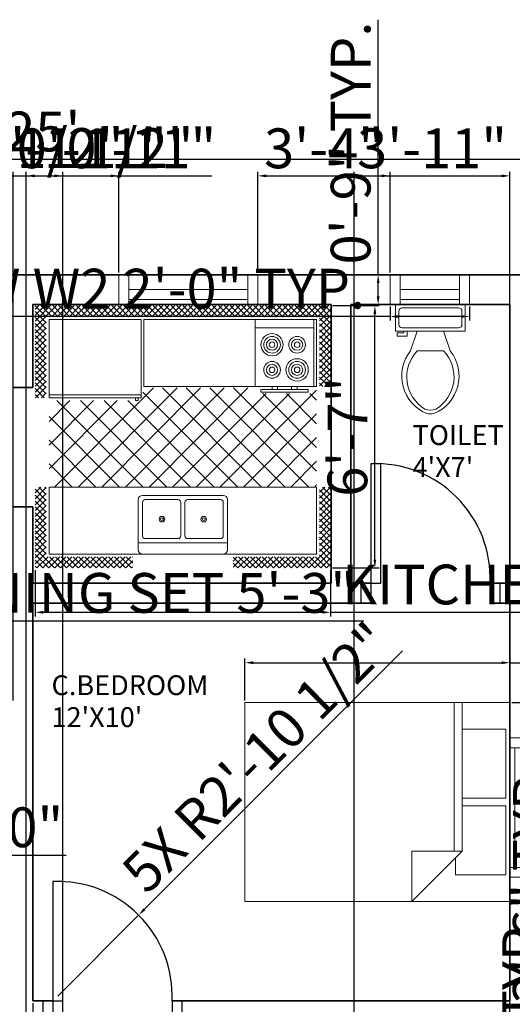
# Model space of a CAD drawing. Units: inches. Extents: x 2011 to 2548, y 530 to 1188.
# Tile 4 of 5: x 2220 to 2368, y 891 to 1188. Entities that reach past the tile are written whole.
import ezdxf

# ---------------------------------------------------------------- set-up
doc = ezdxf.new("R2010")
doc.units = ezdxf.units.IN
for name, color, linetype, lineweight in [('A-ANNO-DIMS', 2, 'Continuous', 18), ('A-AREA-IDEN', 7, 'Continuous', 25), ('A-DOOR', 3, 'Continuous', 25), ('A-FLOR-FIXT', 9, 'Continuous', 18), ('A-FURN', 8, 'Continuous', 18), ('A-GLAZ', 4, 'Continuous', 18), ('A-WALL', 7, 'Continuous', 35)]:
    doc.layers.add(name, color=color, linetype=linetype, lineweight=lineweight)
doc.styles.get("Standard").update_dxf_attribs({"font": 'arial.ttf'})
doc.dimstyles.new('ISO-25', dxfattribs={"dimtxt": 12, "dimasz": 2.5, "dimexe": 1.25, "dimexo": 0.625, "dimtad": 1, "dimdec": 1, "dimlunit": 3, "dimtxsty": 'Standard', "dimcen": 2.5, "dimadec": 0, "dimazin": 0, "dimtfac": 1, "dimtdec": 1, "dimtmove": 0, "dimatfit": 3, "dimfxl": 1, "dimarcsym": 0})

# ---------------------------------------------------------------- blocks, each defined once
blk = doc.blocks.new('Kitchen Layout - 7 x 8 ft')
for p, q in [((-5, 81.32), (2.68, 89)), ((-5, 83.44), (0.56, 89)), ((-5, 85.56), (-1.56, 89)), ((-5, 87.68), (-3.68, 89)), ((-1, 84.97), (-5, 88.97)), ((1.09, 85), (-2.91, 89)), ((3.21, 85), (-0.79, 89)), ((0.81, 85), (4.81, 89)), ((5.34, 85), (1.34, 89)), ((2.93, 85), (6.93, 89)), ((7.46, 85), (3.46, 89)), ((5.05, 85), (9.05, 89)), ((9.58, 85), (5.58, 89)), ((7.17, 85), (11.17, 89)), ((11.7, 85), (7.7, 89)), ((9.29, 85), (13.29, 89)), ((13.82, 85), (9.82, 89)), ((11.41, 85), (15.41, 89)), ((15.94, 85), (11.94, 89)), ((13.53, 85), (17.53, 89)), ((18.06, 85), (14.06, 89)), ((15.65, 85), (19.65, 89)), ((20.18, 85), (16.18, 89)), ((17.78, 85), (21.78, 89)), ((22.31, 85), (18.31, 89)), ((19.9, 85), (23.9, 89)), ((24.43, 85), (20.43, 89)), ((22.02, 85), (26.02, 89)), ((26.55, 85), (22.55, 89)), ((24.14, 85), (28.14, 89)), ((28.67, 85), (24.67, 89)), ((26.26, 85), (30.26, 89)), ((30.79, 85), (26.79, 89)), ((28.38, 85), (32.38, 89)), ((32.91, 85), (28.91, 89)), ((30.5, 85), (34.5, 89)), ((35.03, 85), (31.03, 89)), ((32.63, 85), (36.63, 89)), ((37.16, 85), (33.16, 89)), ((34.75, 85), (38.75, 89)), ((39.28, 85), (35.28, 89)), ((36.87, 85), (40.87, 89)), ((41.4, 85), (37.4, 89)), ((38.99, 85), (42.99, 89)), ((43.52, 85), (39.52, 89)), ((41.11, 85), (45.11, 89)), ((45.64, 85), (41.64, 89)), ((43.23, 85), (47.23, 89)), ((47.76, 85), (43.76, 89)), ((45.35, 85), (49.35, 89)), ((49.88, 85), (45.88, 89)), ((47.47, 85), (51.47, 89)), ((52, 85), (48, 89)), ((49.6, 85), (53.6, 89)), ((54.13, 85), (50.13, 89)), ((51.72, 85), (55.72, 89)), ((56.25, 85), (52.25, 89)), ((53.84, 85), (57.84, 89)), ((58.37, 85), (54.37, 89)), ((55.96, 85), (59.96, 89)), ((60.49, 85), (56.49, 89)), ((58.08, 85), (62.08, 89)), ((62.61, 85), (58.61, 89)), ((60.2, 85), (64.2, 89)), ((64.73, 85), (60.73, 89)), ((62.32, 85), (66.32, 89)), ((66.85, 85), (62.85, 89)), ((64.45, 85), (68.45, 89)), ((68.97, 85), (64.97, 89)), ((66.57, 85), (70.57, 89)), ((71.1, 85), (67.1, 89)), ((68.69, 85), (72.69, 89)), ((73.22, 85), (69.22, 89)), ((70.81, 85), (74.81, 89)), ((75.34, 85), (71.34, 89)), ((72.93, 85), (76.93, 89)), ((77.46, 85), (73.46, 89)), ((75.05, 85), (79.05, 89)), ((79.58, 85), (75.58, 89)), ((77.17, 85), (81.17, 89)), ((81.7, 85), (77.7, 89)), ((79.29, 85), (83.29, 89)), ((83.82, 85), (79.82, 89)), ((81.42, 85), (85.42, 89)), ((85.95, 85), (81.95, 89)), ((83.54, 85), (87.54, 89)), ((88.07, 85), (84.07, 89)), ((85.66, 85), (89.66, 89)), ((90.19, 85), (86.19, 89)), ((87.78, 85), (91.78, 89)), ((92.31, 85), (88.31, 89)), ((89.9, 85), (93.9, 89)), ((94.43, 85), (90.43, 89)), ((92.02, 85), (96.02, 89)), ((96.55, 85), (92.55, 89)), ((94.14, 85), (98.14, 89)), ((101, 82.67), (94.67, 89)), ((96.27, 85), (100.27, 89)), ((101, 84.79), (96.79, 89)), ((101, 86.92), (98.92, 89)), ((-1, 82.85), (-5, 86.85)), ((-1, 80.73), (-5, 84.73)), ((97, 83.61), (101, 87.61)), ((97, 81.49), (101, 85.49)), ((-5, 79.19), (-1, 83.19)), ((-1, 78.61), (-5, 82.61)), ((34, 84), (96, 84)), ((34, 60), (34, 84)), ((96, 84), (96, 60)), ((101, 80.55), (97, 84.55)), ((97, 79.37), (101, 83.37)), ((101, 78.43), (97, 82.43)), ((97, 77.25), (101, 81.25)), ((-5, 77.07), (-1, 81.07)), ((-1, 76.49), (-5, 80.49)), ((-5, 74.95), (-1, 78.95)), ((-1, 74.36), (-5, 78.36)), ((74, 81), (95, 81)), ((101, 76.31), (97, 80.31)), ((97, 75.13), (101, 79.13)), ((101, 74.19), (97, 78.19)), ((-5, 72.83), (-1, 76.83)), ((-1, 72.24), (-5, 76.24)), ((-5, 70.71), (-1, 74.71)), ((-1, 70.12), (-5, 74.12)), ((97, 73.01), (101, 77.01)), ((101, 72.07), (97, 76.07)), ((97, 70.89), (101, 74.89)), ((-5, 68.59), (-1, 72.59)), ((-1, 68), (-5, 72)), ((101, 69.95), (97, 73.95)), ((97, 68.76), (101, 72.76)), ((101, 67.82), (97, 71.82)), ((97, 66.64), (101, 70.64)), ((-5, 66.47), (-1, 70.47)), ((-1, 65.88), (-5, 69.88)), ((-5, 64.35), (-1, 68.35)), ((-1, 63.76), (-5, 67.76)), ((101, 65.7), (97, 69.7)), ((97, 64.52), (101, 68.52)), ((101, 63.58), (97, 67.58)), ((-5, 62.22), (-1, 66.22)), ((-1, 61.64), (-5, 65.64)), ((-5, 60.1), (-1, 64.1)), ((97, 62.4), (101, 66.4)), ((101, 61.46), (97, 65.46)), ((97, 60.28), (101, 64.28)), ((-1, 59.52), (-5, 63.52)), ((-5, 57.98), (-1, 61.98)), ((-1, 57.39), (-5, 61.39)), ((96, 60), (34, 60)), ((80, 60), (80, 59)), ((82, 59), (82, 60)), ((87, 59), (87, 60)), ((89, 60), (89, 59)), ((100.34, 60), (97, 63.34)), ((98.22, 60), (97, 61.22)), ((98.84, 60), (101, 62.16)), ((100.96, 60), (101, 60.04)), ((-1.73, 56), (-5, 59.27)), ((-3.85, 56), (-5, 57.15)), ((-4.86, 56), (-1, 59.86)), ((-2.74, 56), (-1, 57.74)), ((0, 57), (33, 57)), ((10.4, 24), (45.9, 59.5)), ((18.88, 24), (54.38, 59.5)), ((27.37, 24), (62.87, 59.5)), ((33.03, 55.11), (37.41, 59.5)), ((67.71, 24), (33.68, 58.04)), ((35.85, 24), (71.35, 59.5)), ((76.2, 24), (40.7, 59.5)), ((44.34, 24), (77.84, 57.5)), ((84.68, 24), (49.18, 59.5)), ((52.82, 24), (86.32, 57.5)), ((93.17, 24), (57.67, 59.5)), ((61.31, 24), (96, 58.69)), ((96, 29.65), (66.15, 59.5)), ((96, 38.14), (76.64, 57.5)), ((96, 46.63), (85.13, 57.5)), ((96, 55.11), (93.57, 57.54)), ((0, 30.57), (24.43, 55)), ((0, 39.06), (15.94, 55)), ((0, 47.54), (7.46, 55)), ((1.91, 24), (32.91, 55)), ((33.77, 24), (2.77, 55)), ((42.26, 24), (11.26, 55)), ((50.74, 24), (19.74, 55)), ((59.23, 24), (28.23, 55)), ((31, 55), (31, 56)), ((32, 55), (31, 55)), ((32, 56), (32, 55)), ((69.79, 24), (96, 50.21)), ((25.29, 24), (0, 49.29)), ((16.8, 24), (0, 40.8)), ((78.28, 24), (96, 41.72)), ((8.32, 24), (0, 32.32)), ((86.76, 24), (96, 33.24)), ((95.25, 24), (96, 24.75)), ((-5, 21.92), (-2.92, 24)), ((-5, 19.8), (-1, 23.8)), ((-1, 19.21), (-5, 23.21)), ((-5, 17.68), (-1, 21.68)), ((-1, 21.33), (-3.67, 24)), ((-1, 23.45), (-1.55, 24)), ((0, 24), (96, 24)), ((0, 0), (0, 24)), ((96, 24), (96, 0)), ((97, 22.1), (98.9, 24)), ((97, 19.97), (101, 23.97)), ((101, 19.03), (97, 23.03)), ((97, 17.85), (101, 21.85)), ((101, 21.16), (98.16, 24)), ((101, 23.28), (100.28, 24)), ((-1, 17.09), (-5, 21.09)), ((-5, 15.55), (-1, 19.55)), ((-1, 14.97), (-5, 18.97)), ((47.25, 6.5), (47.25, 18.5)), ((48.75, 18.5), (48.75, 6.5)), ((101, 16.91), (97, 20.91)), ((97, 15.73), (101, 19.73)), ((101, 14.79), (97, 18.79)), ((-5, 13.43), (-1, 17.43)), ((-1, 12.85), (-5, 16.85)), ((-5, 11.31), (-1, 15.31)), ((-1, 10.73), (-5, 14.73)), ((97, 13.61), (101, 17.61)), ((101, 12.67), (97, 16.67)), ((97, 11.49), (101, 15.49)), ((101, 10.55), (97, 14.55)), ((-5, 9.19), (-1, 13.19)), ((-1, 8.6), (-5, 12.6)), ((-5, 7.07), (-1, 11.07)), ((97, 9.37), (101, 13.37)), ((101, 8.43), (97, 12.43)), ((97, 7.25), (101, 11.25)), ((-1, 6.48), (-5, 10.48)), ((-5, 4.95), (-1, 8.95)), ((-1, 4.36), (-5, 8.36)), ((101, 6.31), (97, 10.31)), ((97, 5.12), (101, 9.12)), ((101, 4.18), (97, 8.18)), ((-5, 2.83), (-1, 6.83)), ((-1, 2.24), (-5, 6.24)), ((-5, 0.71), (-1, 4.71)), ((-1, 0.12), (-5, 4.12)), ((64, 4), (32, 4)), ((97, 3), (101, 7)), ((101, 2.06), (97, 6.06)), ((97, 0.88), (101, 4.88)), ((101, -0.06), (97, 3.94)), ((-5, -1.42), (-1, 2.58)), ((2, -5), (-5, 2)), ((-5, -3.54), (-1, 0.46)), ((96, 0), (0, 0)), ((93.24, -5), (101, 2.76)), ((95.36, -5), (101, 0.64)), ((101, -2.18), (97, 1.82)), ((-0.12, -5), (-5, -0.12)), ((-2.25, -5), (-5, -2.25)), ((-4.34, -5), (-0.34, -1)), ((-2.22, -5), (1.78, -1)), ((-0.1, -5), (3.9, -1)), ((4.12, -5), (0.12, -1)), ((2.02, -5), (6.02, -1)), ((6.24, -5), (2.24, -1)), ((4.14, -5), (8.14, -1)), ((8.36, -5), (4.36, -1)), ((6.27, -5), (10.27, -1)), ((10.48, -5), (6.48, -1)), ((8.39, -5), (12.39, -1)), ((12.6, -5), (8.6, -1)), ((10.51, -5), (14.51, -1)), ((14.73, -5), (10.73, -1)), ((12.63, -5), (16.63, -1)), ((16.85, -5), (12.85, -1)), ((14.75, -5), (18.75, -1)), ((18.97, -5), (14.97, -1)), ((16.87, -5), (20.87, -1)), ((21.09, -5), (17.09, -1)), ((18.99, -5), (22.99, -1)), ((23.21, -5), (19.21, -1)), ((21.11, -5), (25.11, -1)), ((25.33, -5), (21.33, -1)), ((23.24, -5), (27.24, -1)), ((27.45, -5), (23.45, -1)), ((25.36, -5), (29.36, -1)), ((29.57, -5), (25.57, -1)), ((27.48, -5), (30, -2.48)), ((30, -3.3), (27.7, -1)), ((30, -1.18), (29.82, -1)), ((66, -2.54), (67.54, -1)), ((66, -4.66), (69.66, -1)), ((69.88, -5), (66, -1.12)), ((67.76, -5), (66, -3.24)), ((67.78, -5), (71.78, -1)), ((72, -5), (68, -1)), ((69.9, -5), (73.9, -1)), ((74.12, -5), (70.12, -1)), ((72.03, -5), (76.03, -1)), ((76.24, -5), (72.24, -1)), ((74.15, -5), (78.15, -1)), ((78.36, -5), (74.36, -1)), ((76.27, -5), (80.27, -1)), ((80.49, -5), (76.49, -1)), ((78.39, -5), (82.39, -1)), ((82.61, -5), (78.61, -1)), ((80.51, -5), (84.51, -1)), ((84.73, -5), (80.73, -1)), ((82.63, -5), (86.63, -1)), ((86.85, -5), (82.85, -1)), ((84.75, -5), (88.75, -1)), ((88.97, -5), (84.97, -1)), ((86.88, -5), (90.88, -1)), ((91.09, -5), (87.09, -1)), ((89, -5), (93, -1)), ((93.21, -5), (89.21, -1)), ((91.12, -5), (95.12, -1)), ((95.34, -5), (91.34, -1)), ((97.46, -5), (93.46, -1)), ((99.58, -5), (95.58, -1)), ((101, -4.3), (97, -0.3)), ((97.48, -5), (101, -1.48)), ((-4.37, -5), (-5, -4.37)), ((29.6, -5), (30, -4.6)), ((99.6, -5), (101, -3.6))]:
    blk.add_line(p, q)
for points in [[(0, 56), (0, 84), (33, 84), (33, 56)], [(74, 60), (74, 84), (95, 84), (95, 60)], [(76, 58), (76, 59), (93, 59), (93, 58)]]:
    blk.add_lwpolyline(points, close=True)
for points in [[(32, 1.5), (32, 19.5)], [(33.5, 21), (62.5, 21)], [(33.5, 6.5), (33.5, 18.5)], [(34.5, 19.5), (46.25, 19.5)], [(49.75, 19.5), (61.5, 19.5)], [(62.5, 18.5), (62.5, 6.5)], [(64, 19.5), (64, 1.5)], [(46.25, 5.5), (34.5, 5.5)], [(61.5, 5.5), (49.75, 5.5)], [(62.5, 0), (33.5, 0)]]:
    blk.add_lwpolyline(points)
for centre, radius in [((80, 75), 4), ((80, 75), 3), ((89, 75), 3), ((80, 75), 2), ((80, 75), 1), ((89, 75), 2), ((89, 75), 1), ((80, 66), 3), ((80, 66), 2), ((89, 66), 4), ((89, 66), 3), ((89, 66), 2), ((80, 66), 1), ((89, 66), 1), ((40.5, 12.5), 1), ((40.5, 12.5), 0.5), ((55.5, 12.5), 1), ((55.5, 12.5), 0.5)]:
    blk.add_circle(centre, radius)
for centre, radius, start, end in [((33.5, 19.5), 1.5, 90, 180), ((34.5, 18.5), 1, 90, 180), ((46.25, 18.5), 1, 0, 90), ((49.75, 18.5), 1, 90, 180), ((61.5, 18.5), 1, 0, 90), ((62.5, 19.5), 1.5, 0, 90), ((34.5, 6.5), 1, 180, 270), ((46.25, 6.5), 1, 270, 0), ((49.75, 6.5), 1, 180, 270), ((61.5, 6.5), 1, 270, 0), ((33.5, 1.5), 1.5, 180, 270), ((62.5, 1.5), 1.5, 270, 0)]:
    blk.add_arc(centre, radius, start, end)
blk = doc.blocks.new('Toilet - top')
for p, q in [((9.5, -6), (9.5, -2)), ((-10, -8.5), (-8, -8.5)), ((-10, -9.5), (-10, -8.5)), ((-8, -8.5), (-8, -8)), ((-7, -8), (-7, -9.5)), ((-4, -8), (-6, -14)), ((4, -8), (6, -14)), ((-7, -9.5), (-10, -9.5)), ((4, -14), (-4, -14))]:
    blk.add_line(p, q)
blk.add_lwpolyline([(10.5, -8), (10.5, 0), (-10.5, 0), (-10.5, -8)], close=True)
for points in [[(-9.5, -2), (-9.5, -6)], [(8.5, -1), (-8.5, -1)], [(-8.5, -7), (8.5, -7)]]:
    blk.add_lwpolyline(points)
for centre, radius, start, end in [((-8.62, -1.88), 0.884, 81.8699, 188.1301), ((8.62, -1.88), 0.884, 351.8699, 98.1301), ((-8.62, -6.12), 0.884, 171.8699, 278.1301), ((8.62, -6.12), 0.884, 261.8699, 8.1301), ((3.52, -21.58), 12.17, 141.4691, 247.9714), ((4.2, -21.82), 11.33, 136.3677, 238.9468), ((-3.52, -21.58), 12.17, 292.0284, 38.5307), ((-4.2, -21.82), 11.33, 301.053, 43.6321), ((0, -27.88), 4, 245.7318, 294.2682), ((0, -29), 4, 254.8605, 285.1395)]:
    blk.add_arc(centre, radius, start, end)
blk = doc.blocks.new('Bed - Queen')
for p, q in [((0, -80.00003), (0, 0)), ((0, 0), (59.99999, 0)), ((59.99999, 0), (59.99999, -80.00003)), ((7.99999, -1.2), (28.79998, -1.2)), ((7.99999, -14.4), (7.99999, -1.2)), ((28.79998, -1.2), (28.79998, -14.4)), ((31.19999, -1.2), (51.99999, -1.2)), ((31.19999, -14.4), (31.19999, -1.2)), ((51.99999, -1.2), (51.99999, -16.4)), ((0, -14.4), (44.8, -14.4)), ((59.99999, -29.6), (44.8, -14.4)), ((44.8, -14.4), (44.8, -29.6)), ((44.8, -16.8), (0, -16.8)), ((51.99999, -16.4), (46.79936, -16.4)), ((44.8, -29.6), (59.99999, -29.6)), ((59.99999, -80.00003), (0, -80.00003))]:
    blk.add_line(p, q)
blk = doc.blocks.new('*D12')
at = {"layer": 'A-ANNO-DIMS', "color": 0, "lineweight": -2, "transparency": 16777216}
for p, q in [((2076.53, 1111.98), (2076.53, 1147.49)), ((2079.03, 1146.24), (2374.03, 1146.24)), ((2376.53, 1111.98), (2376.53, 1147.49))]:
    blk.add_line(p, q, dxfattribs=at)
at = {"layer": 'A-ANNO-DIMS', "color": 0, "transparency": 16777216}
for points in [[(2079.03, 1146.66), (2079.03, 1145.82), (2076.53, 1146.24)], [(2374.03, 1146.66), (2374.03, 1145.82), (2376.53, 1146.24)]]:
    blk.add_solid(points, dxfattribs=at)
at = {"layer": 'Defpoints', "color": 0, "transparency": 16777216}
for p in [(2376.53, 1146.24), (2076.53, 1111.36), (2376.53, 1111.36)]:
    blk.add_point(p, dxfattribs=at)
at = {"layer": 'A-ANNO-DIMS', "color": 0, "transparency": 16777216, "insert": (2226.53, 1152.99), "char_height": 12, "attachment_point": 5}
blk.add_mtext("25'", dxfattribs=at)
blk = doc.blocks.new('WIN-36IN')
for p, q in [((0, 42), (9, 42)), ((0, 3), (0, 39)), ((0, 39), (9, 39)), ((1.5, 39), (1.5, 3)), ((4.5, 39), (4.5, 3)), ((9, 39), (9, 3)), ((9, 3), (0, 3)), ((9, 0), (0, 0))]:
    blk.add_line(p, q)
blk = doc.blocks.new('WIN-18IN')
for p, q in [((9, 24), (0, 24)), ((9, 21), (0, 21)), ((0, 21), (0, 3)), ((1.5, 3), (1.5, 21)), ((4.5, 3), (4.5, 21)), ((9, 3), (9, 21)), ((0, 3), (9, 3)), ((0, 0), (9, 0))]:
    blk.add_line(p, q)
blk = doc.blocks.new('DOOR-SWING-36IN-6IN-JAMB')
for p, q in [((0, 6), (0, 0)), ((3, 6), (3, 0)), ((39, 6), (39, 0)), ((42, 6), (42, 0))]:
    blk.add_line(p, q)
blk.add_lwpolyline([(3, 6), (6, 6), (6, 42), (3, 42)], close=True)
blk.add_arc((4.5, 7.5), 34.53, 357.5104, 92.4896)
blk = doc.blocks.new('*D17')
at = {"layer": 'A-ANNO-DIMS', "color": 0, "lineweight": -2, "transparency": 16777216}
for p, q in [((2382.83, 784.45), (2382.83, 969.85)), ((2377.15, 784.45), (2384.08, 784.45)), ((2382.83, 744.95), (2382.83, 781.95)), ((2377.15, 742.45), (2384.08, 742.45))]:
    blk.add_line(p, q, dxfattribs=at)
at = {"layer": 'A-ANNO-DIMS', "color": 0, "transparency": 16777216}
for points in [[(2382.41, 781.95), (2383.24, 781.95), (2382.83, 784.45)], [(2382.41, 744.95), (2383.24, 744.95), (2382.83, 742.45)]]:
    blk.add_solid(points, dxfattribs=at)
at = {"layer": 'Defpoints', "color": 0, "transparency": 16777216}
for p in [(2376.53, 784.45), (2382.83, 784.45), (2376.53, 742.45)]:
    blk.add_point(p, dxfattribs=at)
at = {"layer": 'A-ANNO-DIMS', "color": 0, "transparency": 16777216, "insert": (2375.99, 878.4), "char_height": 12, "attachment_point": 5, "rotation": 90}
blk.add_mtext('WINDOW W1 3\'-6" TYP.', dxfattribs=at)
blk = doc.blocks.new('*D19')
at = {"layer": 'A-ANNO-DIMS', "color": 0, "lineweight": -2, "transparency": 16777216}
for p, q in [((2331.36, 1101.73), (2331.36, 1097.51)), ((2355.36, 1101.73), (2355.36, 1097.51)), ((2331.36, 1098.76), (2145.96, 1098.76)), ((2352.86, 1098.76), (2333.86, 1098.76))]:
    blk.add_line(p, q, dxfattribs=at)
at = {"layer": 'A-ANNO-DIMS', "color": 0, "transparency": 16777216}
for points in [[(2333.86, 1099.18), (2333.86, 1098.34), (2331.36, 1098.76)], [(2352.86, 1099.18), (2352.86, 1098.34), (2355.36, 1098.76)]]:
    blk.add_solid(points, dxfattribs=at)
at = {"layer": 'Defpoints', "color": 0, "transparency": 16777216}
for p in [(2331.36, 1102.36), (2355.36, 1102.36), (2331.36, 1098.76)]:
    blk.add_point(p, dxfattribs=at)
at = {"layer": 'A-ANNO-DIMS', "color": 0, "transparency": 16777216, "insert": (2237.41, 1105.59), "char_height": 12, "attachment_point": 5}
blk.add_mtext('WINDOW W2 2\'-0" TYP.', dxfattribs=at)
blk = doc.blocks.new('*D20')
at = {"layer": 'A-ANNO-DIMS', "color": 0, "lineweight": -2, "transparency": 16777216}
for p, q in [((2327.76, 1111.36), (2327.76, 1188.25)), ((2330.74, 1111.36), (2326.51, 1111.36)), ((2327.76, 1104.86), (2327.76, 1108.86)), ((2330.74, 1102.36), (2326.51, 1102.36))]:
    blk.add_line(p, q, dxfattribs=at)
at = {"layer": 'A-ANNO-DIMS', "color": 0, "transparency": 16777216}
for points in [[(2327.34, 1108.86), (2328.18, 1108.86), (2327.76, 1111.36)], [(2327.34, 1104.86), (2328.18, 1104.86), (2327.76, 1102.36)]]:
    blk.add_solid(points, dxfattribs=at)
at = {"layer": 'Defpoints', "color": 0, "transparency": 16777216}
for p in [(2327.76, 1111.36), (2331.36, 1111.36), (2331.36, 1102.36)]:
    blk.add_point(p, dxfattribs=at)
at = {"layer": 'A-ANNO-DIMS', "color": 0, "transparency": 16777216, "insert": (2321.01, 1151.06), "char_height": 12, "attachment_point": 5, "rotation": 90}
blk.add_mtext('0\'-9" TYP.', dxfattribs=at)
blk = doc.blocks.new('*D23')
at = {"layer": 'A-ANNO-DIMS', "color": 0, "lineweight": -2, "transparency": 16777216}
for p, q in [((2334.48, 872.46), (2334.48, 878.04)), ((2336.98, 876.79), (2365.03, 876.79)), ((2367.53, 872.46), (2367.53, 878.04)), ((2367.53, 876.79), (2477.5, 876.79))]:
    blk.add_line(p, q, dxfattribs=at)
at = {"layer": 'A-ANNO-DIMS', "color": 0, "transparency": 16777216}
for points in [[(2336.98, 877.21), (2336.98, 876.38), (2334.48, 876.79)], [(2365.03, 877.21), (2365.03, 876.38), (2367.53, 876.79)]]:
    blk.add_solid(points, dxfattribs=at)
at = {"layer": 'Defpoints', "color": 0, "transparency": 16777216}
for p in [(2367.53, 876.79), (2334.48, 871.84), (2367.53, 871.84)]:
    blk.add_point(p, dxfattribs=at)
at = {"layer": 'A-ANNO-DIMS', "color": 0, "transparency": 16777216, "insert": (2423.76, 883.62), "char_height": 12, "attachment_point": 5}
blk.add_mtext('WC 2\'-9" TYP.', dxfattribs=at)
blk = doc.blocks.new('*D25')
at = {"layer": 'A-ANNO-DIMS', "color": 0, "lineweight": -2, "transparency": 16777216}
for p, q in [((2287.53, 982.98), (2287.53, 995.61)), ((2367.53, 982.98), (2367.53, 995.61)), ((2290.03, 994.36), (2365.03, 994.36)), ((2367.53, 994.36), (2547.8, 994.36))]:
    blk.add_line(p, q, dxfattribs=at)
at = {"layer": 'A-ANNO-DIMS', "color": 0, "transparency": 16777216}
for points in [[(2290.03, 994.78), (2290.03, 993.94), (2287.53, 994.36)], [(2365.03, 994.78), (2365.03, 993.94), (2367.53, 994.36)]]:
    blk.add_solid(points, dxfattribs=at)
at = {"layer": 'Defpoints', "color": 0, "transparency": 16777216}
for p in [(2367.53, 994.36), (2287.53, 982.36), (2367.53, 982.36)]:
    blk.add_point(p, dxfattribs=at)
at = {"layer": 'A-ANNO-DIMS', "color": 0, "transparency": 16777216, "insert": (2458.91, 1001.56), "char_height": 12, "attachment_point": 5}
blk.add_mtext('QUEEN BED 6\'-8" TYP.', dxfattribs=at)
blk = doc.blocks.new('*D26')
at = {"layer": 'A-ANNO-DIMS', "color": 0, "lineweight": -2, "transparency": 16777216}
for p, q in [((2368.15, 982.36), (2380.78, 982.36)), ((2379.53, 979.86), (2379.53, 924.86)), ((2368.15, 922.36), (2380.78, 922.36)), ((2379.53, 922.36), (2379.53, 845.46))]:
    blk.add_line(p, q, dxfattribs=at)
at = {"layer": 'A-ANNO-DIMS', "color": 0, "transparency": 16777216}
for points in [[(2379.11, 979.86), (2379.94, 979.86), (2379.53, 982.36)], [(2379.11, 924.86), (2379.94, 924.86), (2379.53, 922.36)]]:
    blk.add_solid(points, dxfattribs=at)
at = {"layer": 'Defpoints', "color": 0, "transparency": 16777216}
for p in [(2367.53, 982.36), (2367.53, 922.36), (2379.53, 922.36)]:
    blk.add_point(p, dxfattribs=at)
at = {"layer": 'A-ANNO-DIMS', "color": 0, "transparency": 16777216, "insert": (2372.78, 882.66), "char_height": 12, "attachment_point": 5, "rotation": 90}
blk.add_mtext('5\'-0" TYP.', dxfattribs=at)
blk = doc.blocks.new('*D29')
at = {"layer": 'A-ANNO-DIMS', "color": 0, "lineweight": -2, "transparency": 16777216}
for p, q in [((2224.2, 1022.31), (2224.2, 1008.31)), ((2313.39, 1022.31), (2313.39, 1008.31)), ((2226.7, 1009.56), (2310.89, 1009.56)), ((2313.39, 1009.56), (2426.74, 1009.56))]:
    blk.add_line(p, q, dxfattribs=at)
at = {"layer": 'A-ANNO-DIMS', "color": 0, "transparency": 16777216}
for points in [[(2226.7, 1009.97), (2226.7, 1009.14), (2224.2, 1009.56)], [(2310.89, 1009.97), (2310.89, 1009.14), (2313.39, 1009.56)]]:
    blk.add_solid(points, dxfattribs=at)
at = {"layer": 'Defpoints', "color": 0, "transparency": 16777216}
for p in [(2224.2, 1022.94), (2313.39, 1022.94), (2313.39, 1009.56)]:
    blk.add_point(p, dxfattribs=at)
at = {"layer": 'A-ANNO-DIMS', "color": 0, "transparency": 16777216, "insert": (2371.32, 1016.39), "char_height": 12, "attachment_point": 5}
blk.add_mtext('KITCHEN 7\'-5"', dxfattribs=at)
blk = doc.blocks.new('*D30')
at = {"layer": 'A-ANNO-DIMS', "color": 0, "lineweight": -2, "transparency": 16777216}
for p, q in [((2314.01, 1102.03), (2328.02, 1102.03)), ((2326.77, 1025.44), (2326.77, 1099.53)), ((2314.01, 1022.94), (2328.02, 1022.94))]:
    blk.add_line(p, q, dxfattribs=at)
at = {"layer": 'A-ANNO-DIMS', "color": 0, "transparency": 16777216}
for points in [[(2326.35, 1099.53), (2327.18, 1099.53), (2326.77, 1102.03)], [(2326.35, 1025.44), (2327.18, 1025.44), (2326.77, 1022.94)]]:
    blk.add_solid(points, dxfattribs=at)
at = {"layer": 'Defpoints', "color": 0, "transparency": 16777216}
for p in [(2313.39, 1102.03), (2326.77, 1102.03), (2313.39, 1022.94)]:
    blk.add_point(p, dxfattribs=at)
at = {"layer": 'A-ANNO-DIMS', "color": 0, "transparency": 16777216, "insert": (2320.02, 1062.48), "char_height": 12, "attachment_point": 5, "rotation": 90}
blk.add_mtext('6\'-7"', dxfattribs=at)
blk = doc.blocks.new('*D31')
at = {"layer": 'A-ANNO-DIMS', "color": 0, "lineweight": -2, "transparency": 16777216}
for p, q in [((2088.21, 944.73), (2088.21, 935.11)), ((2148.21, 944.73), (2148.21, 935.11)), ((2090.71, 936.36), (2145.71, 936.36)), ((2148.21, 936.36), (2233.57, 936.36))]:
    blk.add_line(p, q, dxfattribs=at)
at = {"layer": 'A-ANNO-DIMS', "color": 0, "transparency": 16777216}
for points in [[(2090.71, 936.78), (2090.71, 935.94), (2088.21, 936.36)], [(2145.71, 936.78), (2145.71, 935.94), (2148.21, 936.36)]]:
    blk.add_solid(points, dxfattribs=at)
at = {"layer": 'Defpoints', "color": 0, "transparency": 16777216}
for p in [(2088.21, 945.36), (2148.21, 945.36), (2148.21, 936.36)]:
    blk.add_point(p, dxfattribs=at)
at = {"layer": 'A-ANNO-DIMS', "color": 0, "transparency": 16777216, "insert": (2192.14, 943.19), "char_height": 12, "attachment_point": 5}
blk.add_mtext('DESK 5\'-0"', dxfattribs=at)
blk = doc.blocks.new('*D35')
at = {"layer": 'A-ANNO-DIMS', "color": 0, "lineweight": -2, "transparency": 16777216}
for p, q in [((2124.99, 1015.81), (2124.99, 1005.77)), ((2187.78, 1015.81), (2187.78, 1005.77)), ((2127.49, 1007.02), (2185.28, 1007.02)), ((2187.78, 1007.02), (2323.42, 1007.02))]:
    blk.add_line(p, q, dxfattribs=at)
at = {"layer": 'A-ANNO-DIMS', "color": 0, "transparency": 16777216}
for points in [[(2127.49, 1007.44), (2127.49, 1006.6), (2124.99, 1007.02)], [(2185.28, 1007.44), (2185.28, 1006.6), (2187.78, 1007.02)]]:
    blk.add_solid(points, dxfattribs=at)
at = {"layer": 'Defpoints', "color": 0, "transparency": 16777216}
for p in [(2124.99, 1016.44), (2187.78, 1016.44), (2187.78, 1007.02)]:
    blk.add_point(p, dxfattribs=at)
at = {"layer": 'A-ANNO-DIMS', "color": 0, "transparency": 16777216, "insert": (2256.85, 1013.85), "char_height": 12, "attachment_point": 5}
blk.add_mtext('DINING SET 5\'-3"', dxfattribs=at)
blk = doc.blocks.new('*D46')
at = {"layer": 'A-ANNO-DIMS', "color": 0, "lineweight": -2, "transparency": 16777216}
for p, q in [((2221.53, 580.98), (2221.53, 1142.41)), ((2224.03, 1141.16), (2230.03, 1141.16)), ((2232.53, 580.98), (2232.53, 1142.41)), ((2232.53, 1141.16), (2277.5, 1141.16))]:
    blk.add_line(p, q, dxfattribs=at)
at = {"layer": 'A-ANNO-DIMS', "color": 0, "transparency": 16777216}
for points in [[(2224.03, 1141.58), (2224.03, 1140.74), (2221.53, 1141.16)], [(2230.03, 1141.58), (2230.03, 1140.74), (2232.53, 1141.16)]]:
    blk.add_solid(points, dxfattribs=at)
at = {"layer": 'Defpoints', "color": 0, "transparency": 16777216}
for p in [(2232.53, 1141.16), (2221.53, 580.36), (2232.53, 580.36)]:
    blk.add_point(p, dxfattribs=at)
at = {"layer": 'A-ANNO-DIMS', "color": 0, "transparency": 16777216, "insert": (2256.26, 1147.91), "char_height": 12, "attachment_point": 5}
blk.add_mtext('0\'-11"', dxfattribs=at)
blk = doc.blocks.new('*D48')
at = {"layer": 'A-ANNO-DIMS', "color": 0, "lineweight": -2, "transparency": 16777216}
for p, q in [((2178.88, 1111.98), (2178.88, 1142.41)), ((2181.38, 1141.16), (2246.96, 1141.16)), ((2249.46, 1111.98), (2249.46, 1142.41))]:
    blk.add_line(p, q, dxfattribs=at)
at = {"layer": 'A-ANNO-DIMS', "color": 0, "transparency": 16777216}
for points in [[(2181.38, 1141.58), (2181.38, 1140.74), (2178.88, 1141.16)], [(2246.96, 1141.58), (2246.96, 1140.74), (2249.46, 1141.16)]]:
    blk.add_solid(points, dxfattribs=at)
at = {"layer": 'Defpoints', "color": 0, "transparency": 16777216}
for p in [(2249.46, 1141.16), (2178.88, 1111.36), (2249.46, 1111.36)]:
    blk.add_point(p, dxfattribs=at)
at = {"layer": 'A-ANNO-DIMS', "color": 0, "transparency": 16777216, "insert": (2214.17, 1147.99), "char_height": 12, "attachment_point": 5}
blk.add_mtext('5\'-10 1/2"', dxfattribs=at)
blk = doc.blocks.new('*D49')
at = {"layer": 'A-ANNO-DIMS', "color": 0, "lineweight": -2, "transparency": 16777216}
for p, q in [((2291.46, 1111.98), (2291.46, 1142.41)), ((2293.96, 1141.16), (2328.86, 1141.16)), ((2331.36, 1111.98), (2331.36, 1142.41))]:
    blk.add_line(p, q, dxfattribs=at)
at = {"layer": 'A-ANNO-DIMS', "color": 0, "transparency": 16777216}
for points in [[(2293.96, 1141.58), (2293.96, 1140.74), (2291.46, 1141.16)], [(2328.86, 1141.58), (2328.86, 1140.74), (2331.36, 1141.16)]]:
    blk.add_solid(points, dxfattribs=at)
at = {"layer": 'Defpoints', "color": 0, "transparency": 16777216}
for p in [(2331.36, 1141.16), (2291.46, 1111.36), (2331.36, 1111.36)]:
    blk.add_point(p, dxfattribs=at)
at = {"layer": 'A-ANNO-DIMS', "color": 0, "transparency": 16777216, "insert": (2311.41, 1147.91), "char_height": 12, "attachment_point": 5}
blk.add_mtext('3\'-4"', dxfattribs=at)
blk = doc.blocks.new('*D54')
at = {"layer": 'A-ANNO-DIMS', "color": 0, "lineweight": -2, "transparency": 16777216}
for p, q in [((2223.53, 891.73), (2223.53, 540.31)), ((2217.53, 885.73), (2217.53, 540.31)), ((2215.03, 541.56), (2212.53, 541.56)), ((2217.53, 541.56), (2223.53, 541.56)), ((2226.03, 541.56), (2261.68, 541.56))]:
    blk.add_line(p, q, dxfattribs=at)
at = {"layer": 'A-ANNO-DIMS', "color": 0, "transparency": 16777216}
for points in [[(2215.03, 541.98), (2215.03, 541.14), (2217.53, 541.56)], [(2226.03, 541.98), (2226.03, 541.14), (2223.53, 541.56)]]:
    blk.add_solid(points, dxfattribs=at)
at = {"layer": 'Defpoints', "color": 0, "transparency": 16777216}
for p in [(2223.53, 892.36), (2217.53, 886.36), (2223.53, 541.56)]:
    blk.add_point(p, dxfattribs=at)
at = {"layer": 'A-ANNO-DIMS', "color": 0, "transparency": 16777216, "insert": (2245.1, 548.31), "char_height": 12, "attachment_point": 5}
blk.add_mtext('0\'-6"', dxfattribs=at)
blk = doc.blocks.new('*D58')
at = {"layer": 'A-ANNO-DIMS', "color": 0, "lineweight": -2, "transparency": 16777216}
for p, q in [((2157.2, 982.98), (2157.2, 1142.41)), ((2159.7, 1141.16), (2203.98, 1141.16)), ((2206.48, 982.98), (2206.48, 1142.41)), ((2206.48, 1141.16), (2270.57, 1141.16))]:
    blk.add_line(p, q, dxfattribs=at)
at = {"layer": 'A-ANNO-DIMS', "color": 0, "transparency": 16777216}
for points in [[(2159.7, 1141.58), (2159.7, 1140.74), (2157.2, 1141.16)], [(2203.98, 1141.58), (2203.98, 1140.74), (2206.48, 1141.16)]]:
    blk.add_solid(points, dxfattribs=at)
at = {"layer": 'Defpoints', "color": 0, "transparency": 16777216}
for p in [(2206.48, 1141.16), (2157.2, 982.36), (2206.48, 982.36)]:
    blk.add_point(p, dxfattribs=at)
at = {"layer": 'A-ANNO-DIMS', "color": 0, "transparency": 16777216, "insert": (2239.78, 1147.99), "char_height": 12, "attachment_point": 5}
blk.add_mtext('4\'-1 1/2"', dxfattribs=at)
blk = doc.blocks.new('*D59')
at = {"layer": 'A-ANNO-DIMS', "color": 0, "lineweight": -2, "transparency": 16777216}
for p, q in [((2206.48, 982.98), (2206.48, 1142.41)), ((2208.98, 1141.16), (2215.03, 1141.16)), ((2217.53, 982.98), (2217.53, 1142.41)), ((2217.53, 1141.16), (2262.5, 1141.16))]:
    blk.add_line(p, q, dxfattribs=at)
at = {"layer": 'A-ANNO-DIMS', "color": 0, "transparency": 16777216}
for points in [[(2208.98, 1141.58), (2208.98, 1140.74), (2206.48, 1141.16)], [(2215.03, 1141.58), (2215.03, 1140.74), (2217.53, 1141.16)]]:
    blk.add_solid(points, dxfattribs=at)
at = {"layer": 'Defpoints', "color": 0, "transparency": 16777216}
for p in [(2217.53, 1141.16), (2206.48, 982.36), (2217.53, 982.36)]:
    blk.add_point(p, dxfattribs=at)
at = {"layer": 'A-ANNO-DIMS', "color": 0, "transparency": 16777216, "insert": (2241.26, 1147.91), "char_height": 12, "attachment_point": 5}
blk.add_mtext('0\'-11"', dxfattribs=at)
blk = doc.blocks.new('*D60')
at = {"layer": 'A-ANNO-DIMS', "color": 0, "lineweight": -2, "transparency": 16777216}
for p, q in [((2320.53, 580.98), (2320.53, 1142.41)), ((2323.03, 1141.16), (2365.03, 1141.16)), ((2367.53, 580.98), (2367.53, 1142.41))]:
    blk.add_line(p, q, dxfattribs=at)
at = {"layer": 'A-ANNO-DIMS', "color": 0, "transparency": 16777216}
for points in [[(2323.03, 1141.58), (2323.03, 1140.74), (2320.53, 1141.16)], [(2365.03, 1141.58), (2365.03, 1140.74), (2367.53, 1141.16)]]:
    blk.add_solid(points, dxfattribs=at)
at = {"layer": 'Defpoints', "color": 0, "transparency": 16777216}
for p in [(2367.53, 1141.16), (2320.53, 580.36), (2367.53, 580.36)]:
    blk.add_point(p, dxfattribs=at)
at = {"layer": 'A-ANNO-DIMS', "color": 0, "transparency": 16777216, "insert": (2344.03, 1147.91), "char_height": 12, "attachment_point": 5}
blk.add_mtext('3\'-11"', dxfattribs=at)
blk = doc.blocks.new('*D64')
at = {"layer": 'A-ANNO-DIMS', "color": 0, "lineweight": -2, "transparency": 16777216}
for p, q in [((2335.14, 997.97), (2257.21, 920.04)), ((2231.03, 893.86), (2255.45, 918.28))]:
    blk.add_line(p, q, dxfattribs=at)
at = {"layer": 'A-ANNO-DIMS', "color": 0, "transparency": 16777216}
blk.add_solid([(2256.92, 920.34), (2257.51, 919.75), (2255.45, 918.28)], dxfattribs=at)
at = {"layer": 'Defpoints', "color": 0, "transparency": 16777216}
for p in [(2255.45, 918.28), (2231.03, 893.86)]:
    blk.add_point(p, dxfattribs=at)
at = {"layer": 'A-ANNO-DIMS', "color": 0, "transparency": 16777216, "insert": (2292.23, 964.72), "char_height": 12, "attachment_point": 5, "rotation": 45.0003}
blk.add_mtext('5X R2\'-10 1/2"', dxfattribs=at)

msp = doc.modelspace()

# ---------------------------------------------------------------- linework, layer by layer
at = {"layer": 'A-WALL'}
for p, q in [((2223.53, 1102.36), (2223.53, 1077.32)), ((2313.53, 1102.36), (2223.53, 1102.36)), ((2313.53, 1102.36), (2313.53, 1018.36)), ((2367.53, 1102.36), (2319.53, 1102.36)), ((2319.53, 1102.36), (2319.53, 1018.36)), ((2367.53, 1018.36), (2367.53, 1102.36)), ((2217.53, 1077.32), (2223.53, 1077.32)), ((2217.53, 1041.32), (2223.53, 1041.32)), ((2223.53, 1041.32), (2223.53, 1018.36)), ((2313.53, 1018.36), (2223.53, 1018.36)), ((2325.53, 1018.36), (2319.53, 1018.36)), ((2367.53, 1018.36), (2361.53, 1018.36)), ((2223.53, 1012.36), (2223.53, 892.36)), ((2325.53, 1012.36), (2223.53, 1012.36)), ((2367.53, 1012.36), (2361.53, 1012.36)), ((2367.53, 892.36), (2367.53, 1012.36)), ((2229.53, 892.36), (2223.53, 892.36)), ((2367.53, 892.36), (2265.53, 892.36))]:
    msp.add_line(p, q, dxfattribs=at)
msp.add_lwpolyline([(2076.53, 1060.36), (2076.53, 571.36), (2376.53, 571.36), (2376.53, 1111.36), (2076.53, 1111.36), (2076.53, 1096.36)], dxfattribs=at)

# ---------------------------------------------------------------- block references
at = {"layer": 'A-DOOR'}
for p in [(2322.53, 1012.36), (2226.53, 886.36)]:
    msp.add_blockref('DOOR-SWING-36IN-6IN-JAMB', p, dxfattribs=at)
at = {"layer": 'A-FLOR-FIXT', "xscale": 0.8413829192264509, "yscale": 0.8413829192264509, "zscale": 0.8413829192264509}
msp.add_blockref('Kitchen Layout - 7 x 8 ft', (2228.41, 1027.14), dxfattribs=at)
at = {"layer": 'A-FLOR-FIXT'}
msp.add_blockref('Toilet - top', (2343.53, 1102.36), dxfattribs=at)
at = {"layer": 'A-FURN', "rotation": 270}
msp.add_blockref('Bed - Queen', (2367.53, 982.36), dxfattribs=at)
at = {"layer": 'A-GLAZ'}
for name, p, rotation in [('WIN-36IN', (2291.46, 1102.36), 90.00000000000067), ('WIN-18IN', (2355.36, 1102.36), 90.00000000000206)]:
    msp.add_blockref(name, p, dxfattribs=dict(at, rotation=rotation))
msp.add_blockref('WIN-36IN', (2367.53, 929.66), dxfattribs=at)

# ---------------------------------------------------------------- texts
at = {"layer": 'A-AREA-IDEN'}
for s, p in [('TOILET', (2338.15, 1059.99)), ("4'X7'", (2338.15, 1050.35)), ('C.BEDROOM', (2229.14, 984.58)), ("12'X10'", (2229.14, 974.95))]:
    msp.add_text(s, height=6, dxfattribs=at).set_placement(p)

# ---------------------------------------------------------------- dimensions: what is measured, and where the dimension line sits
at = {"layer": 'A-ANNO-DIMS'}
for base, p1, p2, angle, text, picture, middle in [((2327.76, 1111.36), (2331.36, 1102.36), (2331.36, 1111.36), 90, '<> TYP.', '*D20', (2321.01, 1151.06)), ((2331.36, 1098.76), (2355.36, 1102.36), (2331.36, 1102.36), 180, 'WINDOW W2 <> TYP.', '*D19', (2237.41, 1105.59)), ((2379.53, 922.36), (2367.53, 982.36), (2367.53, 922.36), 270, '<> TYP.', '*D26', (2372.78, 882.66)), ((2382.83, 784.45), (2376.53, 742.45), (2376.53, 784.45), 90, 'WINDOW W1 <> TYP.', '*D17', (2375.99, 878.4))]:
    dim = msp.add_linear_dim(base=base, p1=p1, p2=p2, angle=angle, text=text, dimstyle='ISO-25', override={"dimdec": 1, "dimlfac": 1, "dimrnd": 0, "dimzin": 1, "dimdsep": 46, "dimlunit": 4, "dimfrac": 2}, dxfattribs=at)
    dim.commit()
    dim.dimension.update_dxf_attribs({"geometry": picture, "text_midpoint": middle})
for base, p1, p2, override, picture, middle in [((2206.48, 1141.16), (2157.2, 982.36), (2206.48, 982.36), {"dimdec": 1, "dimlfac": 1, "dimrnd": 0, "dimzin": 1, "dimdsep": 46, "dimlunit": 4, "dimfrac": 2}, '*D58', (2239.78, 1147.99)), ((2249.46, 1141.16), (2178.88, 1111.36), (2249.46, 1111.36), {"dimdec": 1, "dimlfac": 1, "dimrnd": 0, "dimzin": 1, "dimdsep": 46, "dimlunit": 4, "dimfrac": 2}, '*D48', (2214.17, 1147.99)), ((2376.53, 1146.24), (2076.53, 1111.36), (2376.53, 1111.36), {"dimclrd": 0, "dimclre": 0, "dimclrt": 0}, '*D12', (2226.53, 1152.99)), ((2217.527, 1141.1587), (2206.4794, 982.3587), (2217.527, 982.3587), {"dimdec": 1, "dimlfac": 1, "dimrnd": 0, "dimzin": 1, "dimdsep": 46, "dimlunit": 4, "dimfrac": 2}, '*D59', (2241.2632, 1147.9106)), ((2232.53, 1141.16), (2221.53, 580.36), (2232.53, 580.36), {"dimdec": 1, "dimlfac": 1, "dimrnd": 0, "dimzin": 1, "dimdsep": 46, "dimlunit": 4, "dimfrac": 2}, '*D46', (2256.26, 1147.91)), ((2331.36, 1141.16), (2291.46, 1111.36), (2331.36, 1111.36), {"dimdec": 1, "dimlfac": 1, "dimrnd": 0, "dimzin": 1, "dimdsep": 46, "dimlunit": 4, "dimfrac": 2}, '*D49', (2311.41, 1147.91)), ((2367.53, 1141.16), (2320.53, 580.36), (2367.53, 580.36), {"dimdec": 1, "dimlfac": 1, "dimrnd": 0, "dimzin": 1, "dimdsep": 46, "dimlunit": 4, "dimfrac": 2}, '*D60', (2344.03, 1147.91)), ((2223.53, 541.56), (2217.53, 886.36), (2223.53, 892.36), {"dimdec": 1, "dimlfac": 1, "dimrnd": 0, "dimzin": 1, "dimdsep": 46, "dimlunit": 4, "dimfrac": 2}, '*D54', (2245.1, 548.31))]:
    dim = msp.add_linear_dim(base=base, p1=p1, p2=p2, dimstyle='ISO-25', override=override, dxfattribs=at)
    dim.commit()
    dim.dimension.update_dxf_attribs({"geometry": picture, "text_midpoint": middle})
dim = msp.add_linear_dim(base=(2326.77, 1102.03), p1=(2313.39, 1022.94), p2=(2313.39, 1102.03), angle=90, dimstyle='ISO-25', override={"dimdec": 1, "dimlfac": 1, "dimrnd": 0, "dimzin": 1, "dimdsep": 46, "dimlunit": 4, "dimfrac": 2}, dxfattribs=at)
dim.commit()
dim.dimension.update_dxf_attribs({"geometry": '*D30', "text_midpoint": (2320.02, 1062.48)})
for base, p1, p2, text, picture, middle in [((2187.78, 1007.02), (2124.99, 1016.44), (2187.78, 1016.44), 'DINING SET <>', '*D35', (2256.85, 1013.85)), ((2367.53, 994.36), (2287.53, 982.36), (2367.53, 982.36), 'QUEEN BED <> TYP.', '*D25', (2458.91, 1001.56)), ((2313.39, 1009.56), (2224.2, 1022.94), (2313.39, 1022.94), 'KITCHEN <>', '*D29', (2371.32, 1016.39)), ((2148.21, 936.36), (2088.21, 945.36), (2148.21, 945.36), 'DESK <>', '*D31', (2192.14, 943.19)), ((2367.527, 876.7924), (2334.4807, 871.8355), (2367.527, 871.8355), 'WC <> TYP.', '*D23', (2423.7639, 883.622))]:
    dim = msp.add_linear_dim(base=base, p1=p1, p2=p2, text=text, dimstyle='ISO-25', override={"dimdec": 1, "dimlfac": 1, "dimrnd": 0, "dimzin": 1, "dimdsep": 46, "dimlunit": 4, "dimfrac": 2}, dxfattribs=at)
    dim.commit()
    dim.dimension.update_dxf_attribs({"geometry": picture, "text_midpoint": middle})
dim = msp.add_radius_dim(center=(2231.03, 893.86), mpoint=(2255.45, 918.28), text='5X <>', dimstyle='ISO-25', override={"dimdec": 1, "dimlfac": 1, "dimrnd": 0, "dimzin": 1, "dimdsep": 46, "dimlunit": 4, "dimfrac": 2}, dxfattribs=at)
dim.commit()
dim.dimension.update_dxf_attribs({"geometry": '*D64', "text_midpoint": (2292.23, 964.72)})

doc.saveas('drawing.dxf')
